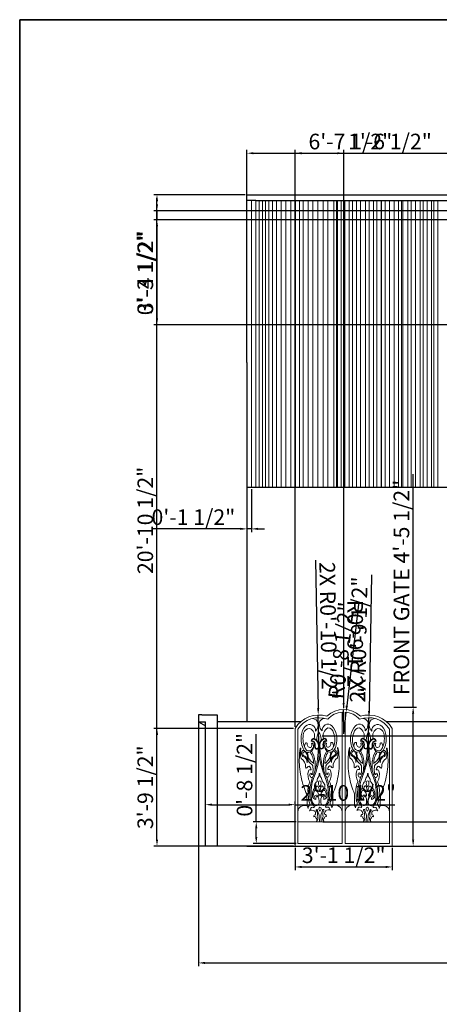
# Model space of a CAD drawing. Units: inches. Extents: x 2656 to 9931, y 1941 to 3068.
# Tile 28 of 46: x 2656 to 2817, y 2689 to 3068. Entities that reach past the tile are written whole.
import ezdxf

# ---------------------------------------------------------------- set-up
doc = ezdxf.new("R2010")
doc.units = ezdxf.units.IN
for name, color, linetype, lineweight in [('A-ANNO-DIMS', 2, 'Continuous', 18), ('A-ANNO-TTLB', 7, 'Continuous', 35), ('A-DOOR', 3, 'Continuous', 18), ('A-ELEV', 7, 'Continuous', 25), ('A-ELEV-FNSH', 8, 'Continuous', 13)]:
    doc.layers.add(name, color=color, linetype=linetype, lineweight=lineweight)
doc.styles.get("Standard").update_dxf_attribs({"font": 'arial.ttf'})
doc.dimstyles.new('ISO-25', dxfattribs={"dimtxt": 6, "dimasz": 2.5, "dimexe": 1.25, "dimexo": 0.625, "dimtad": 1, "dimdec": 0, "dimlunit": 3, "dimtxsty": 'Standard', "dimcen": 2.5, "dimadec": 0, "dimazin": 0, "dimtfac": 1, "dimtdec": 0, "dimtmove": 0, "dimatfit": 3, "dimfxl": 1, "dimarcsym": 0})

# ---------------------------------------------------------------- blocks, each defined once
blk = doc.blocks.new('A$C410F2A13')
for p, q in [((875, 2478), (875, 50)), ((925, 2478), (925, 50)), ((426, 2231), (424, 2281)), ((451, 2231), (449, 2281)), ((1349, 2231), (1351, 2281)), ((1374, 2231), (1376, 2281)), ((0, 2179), (0, 0)), ((50, 2165), (50, 50)), ((1750, 50), (1750, 2165)), ((1800, 0), (1800, 2179)), ((220, 960), (223, 746)), ((697, 967), (700, 754)), ((1103, 967), (1100, 754)), ((1580, 960), (1577, 746)), ((223, 746), (246, 699)), ((700, 754), (679, 706)), ((1100, 754), (1121, 706)), ((1577, 746), (1554, 699)), ((418, 661), (449, 574)), ((449, 574), (450, 450)), ((508, 662), (480, 574)), ((480, 574), (482, 450)), ((1292, 662), (1320, 574)), ((1320, 574), (1318, 450)), ((1351, 574), (1350, 450)), ((1382, 661), (1351, 574)), ((875, 450), (50, 450)), ((1750, 450), (925, 450)), ((1800, 0), (0, 0)), ((875, 50), (50, 50)), ((1750, 50), (925, 50))]:
    blk.add_line(p, q)
for centre, radius, start, end in [((440, 1914), 513, 72.8986, 148.9199), ((440, 1914), 463, 69.1804, 147.2414), ((900, 2081), 448, 46.332, 133.668), ((900, 2081), 398, 93.6017, 137.9637), ((900, 2081), 398, 42.0363, 86.3983), ((1360, 1914), 463, 32.7586, 110.8196), ((1360, 1914), 513, 31.0801, 107.1014), ((404, 2018), 289, 135.8089, 175.1456), ((271, 2143), 108, 353.1272, 134.3061), ((323, 2257), 103, 13.5799, 86.0018), ((283, 2236), 143, 311.7611, 357.9056), ((550, 2260), 103, 95.7845, 168.2064), ((594, 2241), 143, 183.8808, 230.0252), ((609, 2148), 108, 47.4802, 188.6591), ((683, 2044), 163, 118.0779, 198.0674), ((608, 2080), 107, 9.5072, 90.6984), ((433, 2000), 336, 8.9692, 42.4485), ((1367, 2000), 336, 137.5515, 171.0308), ((1192, 2080), 107, 89.3016, 170.4928), ((1191, 2148), 108, 351.3409, 132.5198), ((1117, 2044), 163, 341.9326, 61.9221), ((1250, 2260), 103, 11.7936, 84.2155), ((1206, 2241), 143, 309.9748, 356.1192), ((1517, 2236), 143, 182.0944, 228.2389), ((1477, 2257), 103, 93.9982, 166.4201), ((1529, 2143), 108, 45.6939, 186.8728), ((1396, 2018), 289, 4.8544, 44.1911), ((535, 1983), 424, 171.9264, 209.7222), ((548, 1989), 401, 165.5691, 203.7943), ((274, 2061), 118, 90.9442, 166.1424), ((206, 2037), 157, 343.347, 65.2388), ((652, 1980), 249, 148.1071, 184.9559), ((233, 1973), 249, 356.8304, 33.6792), ((397, 1973), 341, 336.2709, 21.5458), ((368, 1974), 405, 331.6018, 11.2466), ((1432, 1974), 405, 168.7534, 208.3982), ((1403, 1973), 341, 158.4542, 203.7291), ((1567, 1973), 249, 146.3208, 183.1696), ((1148, 1980), 249, 355.0441, 31.8929), ((1594, 2037), 157, 114.7612, 196.653), ((1526, 2061), 118, 13.8576, 89.0558), ((1252, 1989), 401, 336.2057, 14.4309), ((1265, 1983), 424, 330.2778, 8.0736), ((281, 1853), 103, 151.0965, 215.6191), ((208, 1894), 19.8, 343.1885, 153.073), ((277, 1877), 50.8, 167.4858, 297.2236), ((243, 1868), 67.5, 327.8515, 22.0134), ((345, 1949), 44.6, 75.3796, 190.4178), ((303, 1880), 60.3, 355.7551, 91.6639), ((320, 1892), 14.3, 341.4821, 176.919), ((215, 1844), 127, 316.4438, 20.3265), ((219, 1873), 125, 313.8899, 347.6181), ((345, 1949), 33.3, 46.9929, 175.401), ((303, 1880), 71.6, 354.0882, 82.8719), ((296, 1857), 147, 9.4138, 65.971), ((-859, 1778), 1310, 338.6825, 2.2697), ((540, 1859), 178, 174.573, 191.6445), ((405, 1834), 39.9, 195.7675, 306.6665), ((296, 1857), 136, 9.1053, 58.3227), ((540, 1859), 167, 175.2094, 191.4957), ((405, 1834), 28.6, 196.5254, 303.426), ((356, 1855), 78.9, 325.1027, 17.281), ((356, 1855), 90.2, 323.8055, 16.7629), ((1750, 1819), 1310, 179.8498, 203.1038), ((536, 1858), 90.2, 165.0234, 217.9808), ((595, 1862), 147, 115.8153, 172.3725), ((536, 1858), 78.9, 164.5053, 216.6837), ((595, 1862), 136, 123.4636, 172.681), ((488, 1835), 39.9, 235.1198, 346.0188), ((488, 1835), 28.6, 238.3603, 345.2609), ((351, 1856), 167, 350.2906, 6.5769), ((587, 1885), 71.6, 98.9144, 187.6981), ((543, 1952), 33.3, 6.3853, 134.7934), ((351, 1856), 178, 350.1418, 7.2133), ((587, 1885), 60.3, 90.1225, 186.0313), ((543, 1952), 44.6, 351.3685, 106.4067), ((675, 1851), 127, 161.4598, 225.3425), ((670, 1880), 125, 194.1682, 227.8964), ((568, 1896), 14.3, 4.8673, 200.3042), ((645, 1874), 67.5, 159.773, 213.9348), ((611, 1882), 50.8, 244.5627, 14.3005), ((679, 1901), 19.8, 28.7133, 198.5978), ((608, 1858), 103, 326.1672, 30.6898), ((790, 1818), 4.67, 13.9519, 189.3402), ((1010, 1818), 4.67, 350.6598, 166.0481), ((1192, 1858), 103, 149.3102, 213.8328), ((1121, 1901), 19.8, 341.4022, 151.2867), ((1189, 1882), 50.8, 165.6995, 295.4373), ((1155, 1874), 67.5, 326.0652, 20.227), ((1257, 1952), 44.6, 73.5933, 188.6315), ((1213, 1885), 60.3, 353.9687, 89.8775), ((1125, 1851), 127, 314.6575, 18.5402), ((1130, 1880), 125, 312.1036, 345.8318), ((1232, 1896), 14.3, 339.6958, 175.1327), ((1257, 1952), 33.3, 45.2066, 173.6147), ((1213, 1885), 71.6, 352.3019, 81.0856), ((50, 1819), 1310, 336.8962, 0.1502), ((1205, 1862), 147, 7.6275, 64.1847), ((1449, 1856), 178, 172.7867, 189.8582), ((1312, 1835), 39.9, 193.9812, 304.8802), ((1205, 1862), 136, 7.319, 56.5364), ((1449, 1856), 167, 173.4231, 189.7094), ((1312, 1835), 28.6, 194.7391, 301.6397), ((1264, 1858), 78.9, 323.3163, 15.4947), ((1264, 1858), 90.2, 322.0192, 14.9766), ((2659, 1778), 1310, 177.7303, 201.3175), ((1444, 1855), 90.2, 163.2371, 216.1945), ((1504, 1857), 147, 114.029, 170.5862), ((1444, 1855), 78.9, 162.719, 214.8973), ((1504, 1857), 136, 121.6773, 170.8947), ((1395, 1834), 39.9, 233.3335, 344.2325), ((1395, 1834), 28.6, 236.574, 343.4746), ((1260, 1859), 167, 348.5043, 4.7906), ((1497, 1880), 71.6, 97.1281, 185.9118), ((1455, 1949), 33.3, 4.599, 133.0071), ((1260, 1859), 178, 348.3555, 5.427), ((1497, 1880), 60.3, 88.3361, 184.2449), ((1455, 1949), 44.6, 349.5822, 104.6204), ((1585, 1844), 127, 159.6735, 223.5562), ((1581, 1873), 125, 192.3819, 226.1101), ((1480, 1892), 14.3, 3.081, 198.5179), ((1557, 1868), 67.5, 157.9866, 212.1485), ((1523, 1877), 50.8, 242.7764, 12.5142), ((1592, 1894), 19.8, 26.927, 196.8115), ((1519, 1853), 103, 324.3809, 28.9035), ((1612, 1585), 1533, 171.6093, 184.3031), ((100, 1808), 4.67, 352.4461, 167.8344), ((541, 1734), 442, 170.4372, 194.6126), ((203, 1716), 81.7, 156.3863, 223.0742), ((160, 1741), 32.3, 77.4748, 166.6263), ((182, 1708), 40.1, 125.8941, 234.0122), ((120, 1560), 103, 350.7161, 76.6459), ((177, 1718), 29.4, 30.9708, 129.0147), ((137, 1589), 89.3, 5.6042, 76.0929), ((251, 1839), 107, 218.4659, 256.4745), ((256, 1836), 73, 216.1033, 312.5948), ((86, 1643), 147, 341.991, 37.7938), ((242, 1834), 101, 260.608, 309.4662), ((-8, 1638), 253, 349.0382, 22.4521), ((537, 1793), 328, 207.3657, 234.2277), ((6, 1539), 339, 357.9888, 36.5364), ((-43, 1535), 413, 5.2421, 32.4725), ((-859, 1778), 1288, 338.6825, 1.0491), ((1750, 1819), 1288, 180.5839, 203.1038), ((941, 1550), 413, 149.3138, 176.5442), ((892, 1552), 339, 145.2499, 183.7975), ((354, 1790), 328, 307.5586, 334.4207), ((633, 1842), 73, 229.1915, 325.6831), ((647, 1841), 101, 232.3202, 281.1783), ((904, 1653), 253, 159.3342, 192.7481), ((809, 1654), 147, 143.9925, 199.7953), ((638, 1845), 107, 285.3118, 323.3204), ((760, 1599), 89.3, 105.6934, 176.1821), ((778, 1570), 103, 105.1404, 191.0702), ((716, 1726), 29.4, 52.7716, 150.8155), ((732, 1750), 32.3, 15.16, 104.3116), ((712, 1716), 40.1, 307.7741, 55.8923), ((690, 1723), 81.7, 318.7122, 25.4), ((352, 1731), 442, 347.1737, 11.3491), ((-714, 1549), 1533, 357.4832, 10.177), ((2514, 1549), 1533, 169.823, 182.5168), ((1448, 1731), 442, 168.6509, 192.8263), ((1110, 1723), 81.7, 154.6, 221.2878), ((1068, 1750), 32.3, 75.6884, 164.84), ((1088, 1716), 40.1, 124.1077, 232.2259), ((1022, 1570), 103, 348.9298, 74.8596), ((1040, 1599), 89.3, 3.8179, 74.3066), ((1084, 1726), 29.4, 29.1845, 127.2284), ((1162, 1845), 107, 216.6796, 254.6882), ((1167, 1842), 73, 214.3169, 310.8085), ((991, 1654), 147, 340.2047, 36.0075), ((1153, 1841), 101, 258.8217, 307.6798), ((896, 1653), 253, 347.2519, 20.6658), ((1446, 1790), 328, 205.5793, 232.4414), ((908, 1552), 339, 356.2025, 34.7501), ((859, 1550), 413, 3.4558, 30.6862), ((50, 1819), 1288, 336.8962, 359.4161), ((2659, 1778), 1288, 178.9509, 201.3175), ((1843, 1535), 413, 147.5275, 174.7579), ((1794, 1539), 339, 143.4636, 182.0112), ((1263, 1793), 328, 305.7723, 332.6343), ((1544, 1836), 73, 227.4052, 323.8967), ((1558, 1834), 101, 230.5338, 279.392), ((1808, 1638), 253, 157.5479, 190.9618), ((1714, 1643), 147, 142.2062, 198.009), ((1549, 1839), 107, 283.5255, 321.5341), ((1663, 1589), 89.3, 103.9071, 174.3958), ((1680, 1560), 103, 103.3541, 189.2839), ((1623, 1718), 29.4, 50.9853, 149.0292), ((1640, 1741), 32.3, 13.3737, 102.5252), ((1618, 1708), 40.1, 305.9878, 54.1059), ((1597, 1716), 81.7, 316.9258, 23.6137), ((1259, 1734), 442, 345.3874, 9.5628), ((1700, 1808), 4.67, 12.1656, 187.5539), ((188, 1585), 1533, 355.6969, 8.3907), ((1515, 1588), 1436, 184.7143, 199.6369), ((20, 1472), 176, 356.4272, 58.168), ((211, 1459), 15, 168.6782, 347.0514), ((289, 1544), 66.9, 136.2114, 182.0632), ((276, 1426), 58.2, 104.7242, 150.243), ((355, 1631), 122, 199.5388, 236.1164), ((215, 1415), 81.6, 357.4438, 55.6636), ((252, 1458), 79.7, 3.4811, 64.0466), ((-203, 1415), 537, 351.9282, 5.1024), ((-1131, 1472), 1504, 357.1404, 3.8345), ((2032, 1521), 1504, 177.9518, 184.6459), ((1105, 1436), 537, 176.6839, 189.8581), ((649, 1464), 79.7, 117.7397, 178.3052), ((688, 1423), 81.6, 126.1227, 184.3425), ((541, 1634), 122, 305.6699, 342.2475), ((626, 1432), 58.2, 31.5433, 77.0621), ((610, 1549), 66.9, 359.7232, 45.5749), ((691, 1466), 15, 194.7349, 13.1081), ((881, 1486), 176, 123.6183, 185.3591), ((-788, 1575), 1608, 343.3715, 356.674), ((2588, 1575), 1608, 183.326, 196.6285), ((919, 1486), 176, 354.6409, 56.3817), ((1109, 1466), 15, 166.8919, 345.2651), ((1190, 1549), 66.9, 134.4251, 180.2768), ((1174, 1432), 58.2, 102.9379, 148.4567), ((1259, 1634), 122, 197.7525, 234.3301), ((1112, 1423), 81.6, 355.6575, 53.8773), ((1151, 1464), 79.7, 1.6948, 62.2603), ((695, 1436), 537, 350.1419, 3.3161), ((-232, 1521), 1504, 355.3541, 2.0482), ((2931, 1472), 1504, 176.1655, 182.8596), ((2003, 1415), 537, 174.8976, 188.0718), ((1548, 1458), 79.7, 115.9534, 176.5189), ((1585, 1415), 81.6, 124.3364, 182.5562), ((1445, 1631), 122, 303.8836, 340.4612), ((1524, 1426), 58.2, 29.757, 75.2758), ((1511, 1544), 66.9, 357.9368, 43.7886), ((1589, 1459), 15, 192.9486, 11.3218), ((1780, 1472), 176, 121.832, 183.5728), ((285, 1588), 1436, 340.3631, 355.2857), ((510, 1325), 272, 165.7404, 209.4263), ((282, 1375), 39.5, 68.6283, 153.8782), ((335, 1320), 60.6, 168.2152, 221.9825), ((1112, 984), 838, 157.0956, 187.6467), ((294, 1332), 18.8, 3.4092, 180.1447), ((308, 1293), 23.3, 216.4325, 342.6737), ((1112, 984), 815, 157.0956, 187.6467), ((308, 1329), 6.31, 42.5614, 221.6206), ((311, 1341), 17.8, 245.7105, 355.9064), ((375, 1323), 72.5, 313.9549, 9.9508), ((453, 1336), 6.37, 351.4407, 190.3456), ((531, 1325), 72.5, 171.8355, 227.8314), ((-196, 964), 815, 354.1396, 24.6908), ((-196, 964), 838, 354.1396, 24.6908), ((594, 1346), 17.8, 185.8799, 296.0758), ((598, 1298), 23.3, 199.1126, 325.3538), ((611, 1337), 18.8, 1.6416, 178.3771), ((597, 1334), 6.31, 320.1657, 139.2249), ((622, 1380), 39.5, 27.9081, 113.158), ((571, 1324), 60.6, 319.8038, 13.5711), ((396, 1323), 272, 332.36, 16.0459), ((1404, 1323), 272, 163.9541, 207.64), ((1178, 1380), 39.5, 66.842, 152.0919), ((1996, 964), 838, 155.3092, 185.8604), ((1229, 1324), 60.6, 166.4289, 220.1962), ((1189, 1337), 18.8, 1.6229, 178.3584), ((1996, 964), 815, 155.3092, 185.8604), ((1202, 1298), 23.3, 214.6462, 340.8874), ((1203, 1334), 6.31, 40.7751, 219.8343), ((1206, 1346), 17.8, 243.9242, 354.1201), ((1269, 1325), 72.5, 312.1686, 8.1645), ((1347, 1336), 6.37, 349.6544, 188.5593), ((1425, 1323), 72.5, 170.0492, 226.0451), ((688, 984), 815, 352.3533, 22.9044), ((688, 984), 838, 352.3533, 22.9044), ((1492, 1293), 23.3, 197.3263, 323.5675), ((1489, 1341), 17.8, 184.0936, 294.2895), ((1506, 1332), 18.8, 359.8553, 176.5908), ((1492, 1329), 6.31, 318.3794, 137.4386), ((1518, 1375), 39.5, 26.1218, 111.3717), ((1465, 1320), 60.6, 318.0175, 11.7848), ((1290, 1325), 272, 330.5737, 14.2596), ((1034, 1366), 910, 196.6416, 206.516), ((651, 1026), 412, 156.3521, 186.153), ((460, 1109), 99.3, 121.7041, 214.2648), ((432, 1077), 42.5, 130.9198, 211.0137), ((413, 1099), 13.8, 29.7957, 133.7989), ((543, 1204), 135, 150.4288, 184.5495), ((296, 1026), 152, 352.3578, 31.816), ((548, 1163), 114, 168.6269, 216.6185), ((458, 1185), 22, 10.8248, 177.088), ((359, 1169), 122, 322.7993, 9.2913), ((618, 1031), 152, 149.9703, 189.4285), ((366, 1201), 135, 357.2368, 31.3575), ((499, 1100), 13.8, 47.9874, 151.9906), ((452, 1108), 99.3, 327.5215, 60.0822), ((482, 1078), 42.5, 330.7726, 50.8665), ((264, 1020), 412, 355.6333, 25.4342), ((-228, 1401), 1022, 334.8573, 343.6994), ((2028, 1401), 1022, 196.3006, 205.1427), ((1536, 1020), 412, 154.5658, 184.3667), ((1348, 1108), 99.3, 119.9178, 212.4785), ((1318, 1078), 42.5, 129.1335, 209.2274), ((1301, 1100), 13.8, 28.0094, 132.0126), ((1434, 1201), 135, 148.6425, 182.7632), ((1182, 1031), 152, 350.5715, 30.0297), ((1441, 1169), 122, 170.7087, 217.2007), ((1342, 1185), 22, 2.912, 169.1752), ((1252, 1163), 114, 323.3815, 11.3731), ((1504, 1026), 152, 148.184, 187.6422), ((1257, 1204), 135, 355.4505, 29.5712), ((1387, 1099), 13.8, 46.2011, 150.2043), ((1340, 1109), 99.3, 325.7352, 58.2959), ((1368, 1077), 42.5, 328.9863, 49.0802), ((1149, 1026), 412, 353.847, 23.6479), ((766, 1366), 910, 333.484, 343.3584), ((-1225, 770), 1481, 2.6409, 8.2601), ((514, 961), 194, 154.3669, 193.8901), ((392, 933), 69.6, 195.2601, 265.1721), ((361, 1035), 24.7, 46.0398, 154.5946), ((446, 964), 104, 145.8083, 215.978), ((378, 1011), 22, 40.8296, 145.9256), ((407, 900), 45.3, 101.6882, 175.5), ((451, 879), 66.5, 145.8201, 193.29), ((321, 927), 122, 357.8138, 53.2441), ((510, 1123), 133, 210.7996, 241.8374), ((409, 896), 23.8, 28.136, 121.6978), ((401, 892), 51.9, 35.6248, 94.1694), ((402, 1121), 133, 299.949, 330.9867), ((597, 931), 122, 128.5422, 183.9725), ((518, 894), 51.9, 87.6169, 146.1615), ((510, 898), 23.8, 60.0886, 153.6503), ((538, 1013), 22, 35.8607, 140.9567), ((512, 901), 45.3, 6.2863, 80.0981), ((468, 879), 66.5, 348.4963, 35.9662), ((525, 935), 69.6, 276.6142, 346.5263), ((553, 1038), 24.7, 27.1917, 135.7465), ((471, 965), 104, 325.8083, 35.978), ((403, 960), 194, 347.8962, 27.4194), ((2146, 822), 1481, 173.5262, 179.1454), ((-346, 822), 1481, 0.8546, 6.4738), ((1397, 960), 194, 152.5806, 192.1038), ((1275, 935), 69.6, 193.4737, 263.3858), ((1247, 1038), 24.7, 44.2535, 152.8083), ((1329, 965), 104, 144.022, 214.1917), ((1288, 901), 45.3, 99.9019, 173.7137), ((1262, 1013), 22, 39.0433, 144.1393), ((1332, 879), 66.5, 144.0338, 191.5037), ((1290, 898), 23.8, 26.3497, 119.9114), ((1203, 931), 122, 356.0275, 51.4578), ((1282, 894), 51.9, 33.8385, 92.3831), ((1398, 1121), 133, 209.0133, 240.051), ((1290, 1123), 133, 298.1626, 329.2004), ((1479, 927), 122, 126.7559, 182.1862), ((1399, 892), 51.9, 85.8306, 144.3752), ((1391, 896), 23.8, 58.3022, 151.864), ((1393, 900), 45.3, 4.5, 78.3118), ((1349, 879), 66.5, 346.71, 34.1799), ((1422, 1011), 22, 34.0744, 139.1704), ((1408, 933), 69.6, 274.8279, 344.7399), ((1439, 1035), 24.7, 25.4054, 133.9602), ((1354, 964), 104, 324.022, 34.1917), ((1286, 961), 194, 346.1099, 25.6331), ((3025, 770), 1481, 171.7399, 177.3591), ((178, 627), 128, 69.0706, 176.8846), ((308, 708), 62.6, 122.2779, 188.4961), ((126, 764), 148, 358.7797, 29.7342), ((489, 897), 208, 186.6395, 229.065), ((489, 897), 186, 186.6395, 229.065), ((344, 728), 14.3, 246.7853, 56.0942), ((395, 798), 50.3, 236.3592, 331.1413), ((211, 825), 234, 347.3605, 20.5181), ((710, 833), 234, 161.2682, 194.4258), ((527, 801), 50.3, 210.645, 305.4271), ((430, 896), 186, 312.7213, 355.1469), ((580, 731), 14.3, 125.6921, 295.001), ((430, 896), 208, 312.7213, 355.1469), ((797, 775), 148, 152.0521, 183.0067), ((617, 713), 62.6, 353.2902, 59.5084), ((738, 622), 137, 5.1669, 105.9832), ((1062, 622), 137, 74.0168, 174.8331), ((1183, 713), 62.6, 120.4916, 186.7098), ((1003, 775), 148, 356.9933, 27.9479), ((1370, 896), 208, 184.8531, 227.2787), ((1370, 896), 186, 184.8531, 227.2787), ((1220, 731), 14.3, 244.999, 54.3079), ((1273, 801), 50.3, 234.5729, 329.355), ((1090, 833), 234, 345.5742, 18.7318), ((1589, 825), 234, 159.4819, 192.6395), ((1405, 798), 50.3, 208.8587, 303.6408), ((1311, 897), 186, 310.935, 353.3605), ((1456, 728), 14.3, 123.9058, 293.2147), ((1311, 897), 208, 310.935, 353.3605), ((1674, 764), 148, 150.2658, 181.2203), ((1492, 708), 62.6, 351.5039, 57.7221), ((1622, 627), 128, 3.1154, 110.9294), ((240, 690), 44.7, 310.1016, 354.7847), ((309, 568), 96.9, 61.1389, 114.4638), ((322, 681), 37.3, 63.2668, 172.2295), ((377, 551), 31.2, 88.6919, 191.8345), ((360, 526), 23.2, 351.6032, 126.2426), ((319, 603), 62.5, 340.859, 53.3331), ((406, 663), 12.7, 349.8969, 198.3449), ((302, 590), 115, 338.9282, 37.0597), ((354, 505), 70.4, 316.5398, 37.6736), ((462, 695), 23.7, 13.2533, 176.8954), ((503, 699), 64.1, 181.769, 232.1167), ((411, 701), 74.6, 314.8438, 359.9081), ((577, 508), 70.4, 144.1128, 225.2465), ((520, 665), 12.7, 343.4414, 191.8894), ((627, 595), 115, 144.7267, 202.8581), ((609, 607), 62.5, 128.4533, 200.9273), ((570, 529), 23.2, 55.5438, 190.1831), ((553, 554), 31.2, 349.9518, 93.0944), ((620, 573), 96.9, 67.3225, 120.6474), ((604, 686), 37.3, 9.5569, 118.5195), ((685, 697), 44.7, 187.0016, 231.6847), ((1115, 697), 44.7, 308.3153, 352.9984), ((1180, 573), 96.9, 59.3526, 112.6775), ((1196, 686), 37.3, 61.4805, 170.4431), ((1247, 554), 31.2, 86.9056, 190.0482), ((1230, 529), 23.2, 349.8169, 124.4562), ((1191, 607), 62.5, 339.0727, 51.5467), ((1280, 665), 12.7, 348.1106, 196.5586), ((1173, 595), 115, 337.1419, 35.2733), ((1223, 508), 70.4, 314.7535, 35.8872), ((1338, 695), 23.7, 3.1046, 166.7467), ((1389, 701), 74.6, 180.0919, 225.1562), ((1297, 699), 64.1, 307.8833, 358.231), ((1446, 505), 70.4, 142.3264, 223.4602), ((1394, 663), 12.7, 341.6551, 190.1031), ((1498, 590), 115, 142.9403, 201.0718), ((1440, 526), 23.2, 53.7574, 188.3968), ((1481, 603), 62.5, 126.6669, 199.141), ((1423, 551), 31.2, 348.1655, 91.3081), ((1491, 568), 96.9, 65.5362, 118.8611), ((1478, 681), 37.3, 7.7705, 116.7332), ((1560, 690), 44.7, 185.2153, 229.8984), ((356, 484), 47.1, 328.1103, 55.2335), ((401, 458), 4.38, 168.7041, 339.394), ((575, 487), 47.1, 126.5529, 213.676), ((532, 460), 4.38, 202.3923, 13.0822), ((1225, 487), 47.1, 326.324, 53.4471), ((1268, 460), 4.38, 166.9178, 337.6077), ((1399, 458), 4.38, 200.606, 11.2959), ((1444, 484), 47.1, 124.7665, 211.8897)]:
    blk.add_arc(centre, radius, start, end)
blk = doc.blocks.new('*D63')
at = {"layer": 'A-ANNO-DIMS', "color": 0, "lineweight": -2, "transparency": 16777216}
for p, q in [((2807.09, 2803.32), (2807.09, 2893)), ((2799.7, 2803.32), (2808.34, 2803.32)), ((2807.09, 2752.39), (2807.09, 2800.82)), ((2799.7, 2749.89), (2808.34, 2749.89))]:
    blk.add_line(p, q, dxfattribs=at)
at = {"layer": 'A-ANNO-DIMS', "color": 0, "transparency": 16777216}
for points in [[(2806.67, 2800.82), (2807.5, 2800.82), (2807.09, 2803.32)], [(2806.67, 2752.39), (2807.5, 2752.39), (2807.09, 2749.89)]]:
    blk.add_solid(points, dxfattribs=at)
at = {"layer": 'Defpoints', "color": 0, "transparency": 16777216}
for p in [(2799.07, 2803.32), (2807.09, 2803.32), (2799.07, 2749.89)]:
    blk.add_point(p, dxfattribs=at)
at = {"layer": 'A-ANNO-DIMS', "color": 0, "transparency": 16777216, "insert": (2803.36, 2849.41), "char_height": 6, "attachment_point": 5, "rotation": 90}
blk.add_mtext('FRONT GATE 4\'-5 1/2"', dxfattribs=at)
blk = doc.blocks.new('*D64')
at = {"layer": 'A-ANNO-DIMS', "color": 0, "lineweight": -2, "transparency": 16777216}
for p, q in [((2761.66, 2749.27), (2761.66, 2740.63)), ((2799.07, 2749.27), (2799.07, 2740.63)), ((2764.16, 2741.88), (2796.57, 2741.88))]:
    blk.add_line(p, q, dxfattribs=at)
at = {"layer": 'A-ANNO-DIMS', "color": 0, "transparency": 16777216}
for points in [[(2764.16, 2742.3), (2764.16, 2741.46), (2761.66, 2741.88)], [(2796.57, 2742.3), (2796.57, 2741.46), (2799.07, 2741.88)]]:
    blk.add_solid(points, dxfattribs=at)
at = {"layer": 'Defpoints', "color": 0, "transparency": 16777216}
for p in [(2761.66, 2749.89), (2799.07, 2749.89), (2799.07, 2741.88)]:
    blk.add_point(p, dxfattribs=at)
at = {"layer": 'A-ANNO-DIMS', "color": 0, "transparency": 16777216, "insert": (2780.37, 2745.61), "char_height": 6, "attachment_point": 5}
blk.add_mtext('3\'-1 1/2"', dxfattribs=at)
blk = doc.blocks.new('*D77')
at = {"layer": 'A-ANNO-DIMS', "color": 0, "lineweight": -2, "transparency": 16777216}
for p, q in [((2724.52, 2799.77), (2724.52, 2703.71)), ((3030.16, 2801), (3030.16, 2703.71)), ((2727.02, 2704.96), (3027.66, 2704.96))]:
    blk.add_line(p, q, dxfattribs=at)
at = {"layer": 'A-ANNO-DIMS', "color": 0, "transparency": 16777216}
for points in [[(2727.02, 2705.38), (2727.02, 2704.54), (2724.52, 2704.96)], [(3027.66, 2705.38), (3027.66, 2704.54), (3030.16, 2704.96)]]:
    blk.add_solid(points, dxfattribs=at)
at = {"layer": 'Defpoints', "color": 0, "transparency": 16777216}
for p in [(2724.52, 2800.4), (3030.16, 2801.62), (3030.16, 2704.96)]:
    blk.add_point(p, dxfattribs=at)
at = {"layer": 'A-ANNO-DIMS', "color": 0, "transparency": 16777216, "insert": (2877.34, 2708.69), "char_height": 6, "attachment_point": 5}
blk.add_mtext('25\'-5 1/2"', dxfattribs=at)
blk = doc.blocks.new('*D78')
at = {"layer": 'A-ANNO-DIMS', "color": 0, "lineweight": -2, "transparency": 16777216}
for p, q in [((2742.53, 3000.52), (2707.32, 3000.52)), ((2708.57, 2752.39), (2708.57, 2998.02)), ((2726.57, 2749.89), (2707.32, 2749.89))]:
    blk.add_line(p, q, dxfattribs=at)
at = {"layer": 'A-ANNO-DIMS', "color": 0, "transparency": 16777216}
for points in [[(2708.16, 2998.02), (2708.99, 2998.02), (2708.57, 3000.52)], [(2708.16, 2752.39), (2708.99, 2752.39), (2708.57, 2749.89)]]:
    blk.add_solid(points, dxfattribs=at)
at = {"layer": 'Defpoints', "color": 0, "transparency": 16777216}
for p in [(2708.57, 3000.52), (2743.16, 3000.52), (2727.19, 2749.89)]:
    blk.add_point(p, dxfattribs=at)
at = {"layer": 'A-ANNO-DIMS', "color": 0, "transparency": 16777216, "insert": (2704.85, 2875.21), "char_height": 6, "attachment_point": 5, "rotation": 90}
blk.add_mtext('20\'-10 1/2"', dxfattribs=at)
blk = doc.blocks.new('*D83')
at = {"layer": 'A-ANNO-DIMS', "color": 0, "lineweight": -2, "transparency": 16777216}
for p, q in [((2743.16, 2998.91), (2743.16, 3017.72)), ((2745.66, 3016.47), (2820.21, 3016.47)), ((2822.71, 2998.91), (2822.71, 3017.72))]:
    blk.add_line(p, q, dxfattribs=at)
at = {"layer": 'A-ANNO-DIMS', "color": 0, "transparency": 16777216}
for points in [[(2745.66, 3016.88), (2745.66, 3016.05), (2743.16, 3016.47)], [(2820.21, 3016.88), (2820.21, 3016.05), (2822.71, 3016.47)]]:
    blk.add_solid(points, dxfattribs=at)
at = {"layer": 'Defpoints', "color": 0, "transparency": 16777216}
for p in [(2822.71, 3016.47), (2743.16, 2998.29), (2822.71, 2998.29)]:
    blk.add_point(p, dxfattribs=at)
at = {"layer": 'A-ANNO-DIMS', "color": 0, "transparency": 16777216, "insert": (2782.93, 3020.19), "char_height": 6, "attachment_point": 5}
blk.add_mtext('6\'-7 1/2"', dxfattribs=at)
blk = doc.blocks.new('*D88')
at = {"layer": 'A-ANNO-DIMS', "color": 0, "lineweight": -2, "transparency": 16777216}
for p, q in [((2727.19, 2750.52), (2727.19, 2767.09)), ((2729.69, 2765.84), (2759.16, 2765.84)), ((2761.66, 2750.52), (2761.66, 2767.09)), ((2761.66, 2765.84), (2800.1, 2765.84))]:
    blk.add_line(p, q, dxfattribs=at)
at = {"layer": 'A-ANNO-DIMS', "color": 0, "transparency": 16777216}
for points in [[(2729.69, 2766.26), (2729.69, 2765.43), (2727.19, 2765.84)], [(2759.16, 2766.26), (2759.16, 2765.43), (2761.66, 2765.84)]]:
    blk.add_solid(points, dxfattribs=at)
at = {"layer": 'Defpoints', "color": 0, "transparency": 16777216}
for p in [(2761.66, 2765.84), (2727.19, 2749.89), (2761.66, 2749.89)]:
    blk.add_point(p, dxfattribs=at)
at = {"layer": 'A-ANNO-DIMS', "color": 0, "transparency": 16777216, "insert": (2782.13, 2769.57), "char_height": 6, "attachment_point": 5}
blk.add_mtext('2\'-10 1/2"', dxfattribs=at)
blk = doc.blocks.new('*D152')
at = {"layer": 'A-ANNO-DIMS', "color": 0, "lineweight": -2, "transparency": 16777216}
for p, q in [((2847.28, 2990.83), (2707.32, 2990.83)), ((2708.57, 2988.33), (2708.57, 2952.97)), ((2847.25, 2950.47), (2707.32, 2950.47))]:
    blk.add_line(p, q, dxfattribs=at)
at = {"layer": 'A-ANNO-DIMS', "color": 0, "transparency": 16777216}
for points in [[(2708.16, 2988.33), (2708.99, 2988.33), (2708.57, 2990.83)], [(2708.16, 2952.97), (2708.99, 2952.97), (2708.57, 2950.47)]]:
    blk.add_solid(points, dxfattribs=at)
at = {"layer": 'Defpoints', "color": 0, "transparency": 16777216}
for p in [(2847.9, 2990.83), (2708.57, 2950.47), (2847.87, 2950.47)]:
    blk.add_point(p, dxfattribs=at)
at = {"layer": 'A-ANNO-DIMS', "color": 0, "transparency": 16777216, "insert": (2704.84, 2970.65), "char_height": 6, "attachment_point": 5, "rotation": 90}
blk.add_mtext('3\'-4 1/2"', dxfattribs=at)
blk = doc.blocks.new('*D154')
at = {"layer": 'A-ANNO-DIMS', "color": 0, "lineweight": -2, "transparency": 16777216}
for p, q in [((2708.57, 2996.85), (2708.57, 2999.35)), ((2826.02, 2994.35), (2707.32, 2994.35)), ((2708.57, 2994.35), (2708.57, 2990.83)), ((2847.28, 2990.83), (2707.32, 2990.83)), ((2708.57, 2988.33), (2708.57, 2954.65))]:
    blk.add_line(p, q, dxfattribs=at)
at = {"layer": 'A-ANNO-DIMS', "color": 0, "transparency": 16777216}
for points in [[(2708.16, 2996.85), (2708.99, 2996.85), (2708.57, 2994.35)], [(2708.16, 2988.33), (2708.99, 2988.33), (2708.57, 2990.83)]]:
    blk.add_solid(points, dxfattribs=at)
at = {"layer": 'Defpoints', "color": 0, "transparency": 16777216}
for p in [(2826.64, 2994.35), (2708.57, 2990.83), (2847.9, 2990.83)]:
    blk.add_point(p, dxfattribs=at)
at = {"layer": 'A-ANNO-DIMS', "color": 0, "transparency": 16777216, "insert": (2704.84, 2970.24), "char_height": 6, "attachment_point": 5, "rotation": 90}
blk.add_mtext('0\'-3 1/2"', dxfattribs=at)
blk = doc.blocks.new('*D155')
at = {"layer": 'A-ANNO-DIMS', "color": 0, "lineweight": -2, "transparency": 16777216}
for p, q in [((2743.16, 2887.27), (2743.16, 2870.69)), ((2744.89, 2887.27), (2744.89, 2870.69)), ((2740.66, 2871.94), (2706.98, 2871.94)), ((2744.89, 2871.94), (2743.16, 2871.94)), ((2747.39, 2871.94), (2749.89, 2871.94))]:
    blk.add_line(p, q, dxfattribs=at)
at = {"layer": 'A-ANNO-DIMS', "color": 0, "transparency": 16777216}
for points in [[(2740.66, 2872.36), (2740.66, 2871.53), (2743.16, 2871.94)], [(2747.39, 2872.36), (2747.39, 2871.53), (2744.89, 2871.94)]]:
    blk.add_solid(points, dxfattribs=at)
at = {"layer": 'Defpoints', "color": 0, "transparency": 16777216}
for p in [(2743.16, 2887.89), (2744.89, 2887.89), (2743.16, 2871.94)]:
    blk.add_point(p, dxfattribs=at)
at = {"layer": 'A-ANNO-DIMS', "color": 0, "transparency": 16777216, "insert": (2722.57, 2875.67), "char_height": 6, "attachment_point": 5}
blk.add_mtext('0\'-1 1/2"', dxfattribs=at)
blk = doc.blocks.new('*D169')
at = {"layer": 'A-ANNO-DIMS', "color": 0, "lineweight": -2, "transparency": 16777216}
for p, q in [((2761.03, 2795.19), (2707.32, 2795.19)), ((2708.57, 2752.39), (2708.57, 2792.69)), ((2761.03, 2749.89), (2707.32, 2749.89))]:
    blk.add_line(p, q, dxfattribs=at)
at = {"layer": 'A-ANNO-DIMS', "color": 0, "transparency": 16777216}
for points in [[(2708.16, 2792.69), (2708.99, 2792.69), (2708.57, 2795.19)], [(2708.16, 2752.39), (2708.99, 2752.39), (2708.57, 2749.89)]]:
    blk.add_solid(points, dxfattribs=at)
at = {"layer": 'Defpoints', "color": 0, "transparency": 16777216}
for p in [(2708.57, 2795.19), (2761.66, 2795.19), (2761.66, 2749.89)]:
    blk.add_point(p, dxfattribs=at)
at = {"layer": 'A-ANNO-DIMS', "color": 0, "transparency": 16777216, "insert": (2704.84, 2772.54), "char_height": 6, "attachment_point": 5, "rotation": 90}
blk.add_mtext('3\'-9 1/2"', dxfattribs=at)
blk = doc.blocks.new('*D170')
at = {"layer": 'A-ANNO-DIMS', "color": 0, "lineweight": -2, "transparency": 16777216}
for p, q in [((2761.66, 2795.82), (2761.66, 3017.72)), ((2764.16, 3016.47), (2777.87, 3016.47)), ((2780.37, 2803.08), (2780.37, 3017.72)), ((2780.37, 3016.47), (2813.48, 3016.47))]:
    blk.add_line(p, q, dxfattribs=at)
at = {"layer": 'A-ANNO-DIMS', "color": 0, "transparency": 16777216}
for points in [[(2764.16, 3016.88), (2764.16, 3016.05), (2761.66, 3016.47)], [(2777.87, 3016.88), (2777.87, 3016.05), (2780.37, 3016.47)]]:
    blk.add_solid(points, dxfattribs=at)
at = {"layer": 'Defpoints', "color": 0, "transparency": 16777216}
for p in [(2780.37, 3016.47), (2780.37, 2802.46), (2761.66, 2795.19)]:
    blk.add_point(p, dxfattribs=at)
at = {"layer": 'A-ANNO-DIMS', "color": 0, "transparency": 16777216, "insert": (2798.17, 3020.19), "char_height": 6, "attachment_point": 5}
blk.add_mtext('1\'-6 1/2"', dxfattribs=at)
blk = doc.blocks.new('*D171')
at = {"layer": 'A-ANNO-DIMS', "color": 0, "lineweight": -2, "transparency": 16777216}
for p, q in [((2746.75, 2759.25), (2746.75, 2792.93)), ((2762.07, 2759.25), (2745.5, 2759.25)), ((2746.75, 2753.43), (2746.75, 2756.75)), ((2762.07, 2750.93), (2745.5, 2750.93))]:
    blk.add_line(p, q, dxfattribs=at)
at = {"layer": 'A-ANNO-DIMS', "color": 0, "transparency": 16777216}
for points in [[(2746.33, 2756.75), (2747.16, 2756.75), (2746.75, 2759.25)], [(2746.33, 2753.43), (2747.16, 2753.43), (2746.75, 2750.93)]]:
    blk.add_solid(points, dxfattribs=at)
at = {"layer": 'Defpoints', "color": 0, "transparency": 16777216}
for p in [(2746.75, 2759.25), (2762.7, 2759.25), (2762.7, 2750.93)]:
    blk.add_point(p, dxfattribs=at)
at = {"layer": 'A-ANNO-DIMS', "color": 0, "transparency": 16777216, "insert": (2743.02, 2777.34), "char_height": 6, "attachment_point": 5, "rotation": 90}
blk.add_mtext('0\'-8 1/2"', dxfattribs=at)
blk = doc.blocks.new('*D179')
at = {"layer": 'A-ANNO-DIMS', "color": 0, "lineweight": -2, "transparency": 16777216}
for p, q in [((2772.12, 2792.27), (3047.36, 2792.27)), ((3046.11, 2761.76), (3046.11, 2789.77)), ((2772.31, 2759.26), (3047.36, 2759.26))]:
    blk.add_line(p, q, dxfattribs=at)
at = {"layer": 'A-ANNO-DIMS', "color": 0, "transparency": 16777216}
for points in [[(3045.69, 2789.77), (3046.53, 2789.77), (3046.11, 2792.27)], [(3045.69, 2761.76), (3046.53, 2761.76), (3046.11, 2759.26)]]:
    blk.add_solid(points, dxfattribs=at)
at = {"layer": 'Defpoints', "color": 0, "transparency": 16777216}
for p in [(2771.5, 2792.27), (3046.11, 2792.27), (2771.68, 2759.26)]:
    blk.add_point(p, dxfattribs=at)
at = {"layer": 'A-ANNO-DIMS', "color": 0, "transparency": 16777216, "insert": (3042.42, 2775.76), "char_height": 6, "attachment_point": 5, "rotation": 90}
blk.add_mtext('2\'-9"', dxfattribs=at)
blk = doc.blocks.new('*D180')
at = {"layer": 'A-ANNO-DIMS', "color": 0, "lineweight": -2, "transparency": 16777216}
for p, q in [((2780.28, 2844.38), (2780.35, 2804.96)), ((2780.37, 2793.15), (2780.35, 2802.46))]:
    blk.add_line(p, q, dxfattribs=at)
at = {"layer": 'A-ANNO-DIMS', "color": 0, "transparency": 16777216}
blk.add_solid([(2780.76, 2804.96), (2779.93, 2804.96), (2780.35, 2802.46)], dxfattribs=at)
at = {"layer": 'Defpoints', "color": 0, "transparency": 16777216}
for p in [(2780.35, 2802.46), (2780.37, 2793.15)]:
    blk.add_point(p, dxfattribs=at)
at = {"layer": 'A-ANNO-DIMS', "color": 0, "transparency": 16777216, "insert": (2784.04, 2825.93), "char_height": 6, "attachment_point": 5, "rotation": 270.0963}
blk.add_mtext('R0\'-9 1/2"', dxfattribs=at)
blk = doc.blocks.new('*D181')
at = {"layer": 'A-ANNO-DIMS', "color": 0, "lineweight": -2, "transparency": 16777216}
for p, q in [((2769.5, 2859.92), (2770.55, 2802.85)), ((2770.8, 2789.68), (2770.6, 2800.35))]:
    blk.add_line(p, q, dxfattribs=at)
at = {"layer": 'A-ANNO-DIMS', "color": 0, "transparency": 16777216}
blk.add_solid([(2770.97, 2802.86), (2770.14, 2802.85), (2770.6, 2800.35)], dxfattribs=at)
at = {"layer": 'Defpoints', "color": 0, "transparency": 16777216}
for p in [(2770.6, 2800.35), (2770.8, 2789.68)]:
    blk.add_point(p, dxfattribs=at)
at = {"layer": 'A-ANNO-DIMS', "color": 0, "transparency": 16777216, "insert": (2773.73, 2832.71), "char_height": 6, "attachment_point": 5, "rotation": 271.0604}
blk.add_mtext('2X R0\'-10 1/2"', dxfattribs=at)
blk = doc.blocks.new('*D182')
at = {"layer": 'A-ANNO-DIMS', "color": 0, "lineweight": -2, "transparency": 16777216}
for p, q in [((2786.01, 2843.02), (2781.58, 2803.85)), ((2780.37, 2793.15), (2781.3, 2801.37))]:
    blk.add_line(p, q, dxfattribs=at)
at = {"layer": 'A-ANNO-DIMS', "color": 0, "transparency": 16777216}
blk.add_solid([(2781.16, 2803.9), (2781.99, 2803.8), (2781.3, 2801.37)], dxfattribs=at)
at = {"layer": 'Defpoints', "color": 0, "transparency": 16777216}
for p in [(2781.3, 2801.37), (2780.37, 2793.15)]:
    blk.add_point(p, dxfattribs=at)
at = {"layer": 'A-ANNO-DIMS', "color": 0, "transparency": 16777216, "insert": (2780.23, 2825.1), "char_height": 6, "attachment_point": 5, "rotation": 83.5406}
blk.add_mtext('R0\'-8 1/2"', dxfattribs=at)
blk = doc.blocks.new('*D183')
at = {"layer": 'A-ANNO-DIMS', "color": 0, "lineweight": -2, "transparency": 16777216}
for p, q in [((2791.05, 2854.22), (2790.14, 2801.81)), ((2789.93, 2789.68), (2790.1, 2799.31))]:
    blk.add_line(p, q, dxfattribs=at)
at = {"layer": 'A-ANNO-DIMS', "color": 0, "transparency": 16777216}
blk.add_solid([(2789.73, 2801.82), (2790.56, 2801.81), (2790.1, 2799.31)], dxfattribs=at)
at = {"layer": 'Defpoints', "color": 0, "transparency": 16777216}
for p in [(2790.1, 2799.31), (2789.93, 2789.68)]:
    blk.add_point(p, dxfattribs=at)
at = {"layer": 'A-ANNO-DIMS', "color": 0, "transparency": 16777216, "insert": (2786.89, 2829.33), "char_height": 6, "attachment_point": 5, "rotation": 89.0094}
blk.add_mtext('2X R0\'-9 1/2"', dxfattribs=at)

msp = doc.modelspace()

# ---------------------------------------------------------------- linework, layer by layer
at = {"layer": 'A-ANNO-TTLB'}
msp.add_lwpolyline([(2655.77, 3067.84), (3515.43, 3067.84), (3515.43, 1940.89), (2655.77, 1940.89)], close=True, dxfattribs=at)
at = {"layer": 'A-ELEV'}
for p, q in [((2743.16, 2935.89), (2743.16, 3000.52)), ((2743.16, 3000.52), (2884.23, 3000.52)), ((2746.62, 2998.29), (2743.16, 2998.29)), ((2746.62, 2998.29), (2873.91, 2998.29)), ((2743.16, 2935.89), (2743.16, 2797.89)), ((2998.16, 2887.89), (2743.16, 2887.89)), ((2725.77, 2800.4), (2724.52, 2800.4)), ((2724.52, 2800.4), (2724.52, 2797.69)), ((2725.77, 2800.4), (2730.74, 2800.4)), ((2730.74, 2800.4), (2731.73, 2800.4)), ((2731.73, 2800.4), (2731.73, 2749.89)), ((2724.52, 2797.69), (2727.19, 2797.69)), ((2724.52, 2797.69), (2727.19, 2796.13)), ((2727.19, 2749.89), (2727.19, 2797.69)), ((2731.73, 2797.89), (2763.98, 2797.89)), ((2796.75, 2797.89), (3023.35, 2797.89)), ((2728.16, 2749.89), (2727.19, 2749.89)), ((2743.16, 2749.89), (2728.16, 2749.89)), ((2743.16, 2749.89), (2998.16, 2749.89)), ((2743.16, 2749.89), (2998.16, 2749.89))]:
    msp.add_line(p, q, dxfattribs=at)
at = {"layer": 'A-ELEV-FNSH'}
for p, q in [((2744.89, 2887.89), (2744.89, 2998.29)), ((2746.62, 2887.89), (2746.62, 2998.29)), ((2747.86, 2887.89), (2747.86, 2998.29)), ((2749.12, 2887.89), (2749.12, 2998.29)), ((2750.32, 2887.89), (2750.32, 2998.29)), ((2751.62, 2887.89), (2751.62, 2998.29)), ((2753.05, 2887.89), (2753.05, 2998.29)), ((2754.54, 2887.89), (2754.54, 2998.29)), ((2756.31, 2887.89), (2756.31, 2998.29)), ((2758.12, 2887.89), (2758.12, 2998.29)), ((2760.01, 2887.89), (2760.01, 2998.29)), ((2761.79, 2887.89), (2761.79, 2998.29)), ((2763.4, 2887.89), (2763.4, 2998.29)), ((2764.84, 2887.89), (2764.84, 2998.29)), ((2764.84, 2887.89), (2764.84, 2998.29)), ((2766.67, 2887.89), (2766.67, 2998.29)), ((2768.47, 2887.89), (2768.47, 2998.29)), ((2770.49, 2887.89), (2770.49, 2998.29)), ((2772.49, 2887.89), (2772.49, 2998.29)), ((2774.31, 2887.89), (2774.31, 2998.29)), ((2776.53, 2887.89), (2776.53, 2998.29)), ((2777.55, 2887.89), (2777.55, 2998.29)), ((2778.02, 2887.89), (2778.02, 2998.29)), ((2779.46, 2887.89), (2779.46, 2998.29)), ((2780.85, 2887.89), (2780.85, 2998.29)), ((2782.43, 2887.89), (2782.43, 2998.29)), ((2783.76, 2887.89), (2783.76, 2998.29)), ((2785.27, 2887.89), (2785.27, 2998.29)), ((2786.8, 2887.89), (2786.8, 2998.29)), ((2788.76, 2887.89), (2788.76, 2998.29)), ((2790.12, 2887.89), (2790.12, 2998.29)), ((2791.8, 2887.89), (2791.8, 2998.29)), ((2793.1, 2887.89), (2793.1, 2998.29)), ((2794.82, 2887.89), (2794.82, 2998.29)), ((2794.89, 2887.89), (2794.89, 2998.29)), ((2796.3, 2887.89), (2796.3, 2998.29)), ((2797.95, 2887.89), (2797.95, 2998.29)), ((2799.81, 2887.89), (2799.81, 2998.29)), ((2801.41, 2887.89), (2801.41, 2998.29)), ((2802.66, 2887.89), (2802.66, 2998.29)), ((2803.13, 2887.89), (2803.13, 2998.29)), ((2805.11, 2887.89), (2805.11, 2998.29)), ((2806.28, 2887.89), (2806.28, 2998.29)), ((2807.96, 2887.89), (2807.96, 2998.29)), ((2809.79, 2887.89), (2809.79, 2998.29)), ((2810.9, 2887.89), (2810.9, 2998.29)), ((2812.48, 2887.89), (2812.48, 2998.29)), ((2814.11, 2887.89), (2814.11, 2998.29)), ((2815.05, 2887.89), (2815.05, 2998.29)), ((2816.6, 2887.89), (2816.6, 2998.29))]:
    msp.add_line(p, q, dxfattribs=at)

# ---------------------------------------------------------------- block references
at = {"layer": 'A-DOOR', "xscale": 0.0207871243799849, "yscale": 0.0207871243799849, "zscale": 0.0207871243799849}
msp.add_blockref('A$C410F2A13', (2761.66, 2749.89), dxfattribs=at)

# ---------------------------------------------------------------- dimensions: what is measured, and where the dimension line sits
at = {"layer": 'A-ANNO-DIMS'}
for base, p1, p2, picture, middle in [((2822.7053, 3016.4671), (2743.1573, 2998.2859), (2822.7053, 2998.2859), '*D83', (2782.9313, 3020.1944)), ((2780.37, 3016.47), (2761.66, 2795.19), (2780.37, 2802.46), '*D170', (2798.17, 3020.19)), ((3030.16, 2704.96), (2724.52, 2800.4), (3030.16, 2801.62), '*D77', (2877.34, 2708.69)), ((2761.66, 2765.84), (2727.19, 2749.89), (2761.66, 2749.89), '*D88', (2782.13, 2769.57)), ((2799.07, 2741.88), (2761.66, 2749.89), (2799.07, 2749.89), '*D64', (2780.37, 2745.61))]:
    dim = msp.add_linear_dim(base=base, p1=p1, p2=p2, dimstyle='ISO-25', override={"dimdec": 1, "dimlfac": 1, "dimrnd": 0, "dimzin": 1, "dimdsep": 46, "dimlunit": 4, "dimfrac": 2}, dxfattribs=at)
    dim.commit()
    dim.dimension.update_dxf_attribs({"geometry": picture, "text_midpoint": middle})
for base, p1, p2, angle, picture, middle in [((2708.57, 3000.52), (2727.19, 2749.89), (2743.16, 3000.52), 90, '*D78', (2704.85, 2875.21)), ((2708.57, 2990.83), (2826.64, 2994.35), (2847.9, 2990.83), 90, '*D154', (2704.84, 2970.24)), ((2708.57, 2950.47), (2847.9, 2990.83), (2847.87, 2950.47), 90, '*D152', (2704.84, 2970.65)), ((2743.16, 2871.94), (2744.89, 2887.89), (2743.16, 2887.89), 180, '*D155', (2722.57, 2875.67)), ((2708.57, 2795.19), (2761.66, 2749.89), (2761.66, 2795.19), 90, '*D169', (2704.84, 2772.54)), ((2746.75, 2759.25), (2762.7, 2750.93), (2762.7, 2759.25), 90, '*D171', (2743.02, 2777.34)), ((3046.11, 2792.27), (2771.68, 2759.26), (2771.5, 2792.27), 90, '*D179', (3042.42, 2775.76))]:
    dim = msp.add_linear_dim(base=base, p1=p1, p2=p2, angle=angle, dimstyle='ISO-25', override={"dimdec": 1, "dimlfac": 1, "dimrnd": 0, "dimzin": 1, "dimdsep": 46, "dimlunit": 4, "dimfrac": 2}, dxfattribs=at)
    dim.commit()
    dim.dimension.update_dxf_attribs({"geometry": picture, "text_midpoint": middle})
dim = msp.add_linear_dim(base=(2807.09, 2803.32), p1=(2799.07, 2749.89), p2=(2799.07, 2803.32), angle=90, text='FRONT GATE <>', dimstyle='ISO-25', override={"dimdec": 1, "dimlfac": 1, "dimrnd": 0, "dimzin": 1, "dimdsep": 46, "dimlunit": 4, "dimfrac": 2}, dxfattribs=at)
dim.commit()
dim.dimension.update_dxf_attribs({"geometry": '*D63', "text_midpoint": (2803.36, 2849.41)})
for center, mpoint, picture, middle in [((2770.8, 2789.68), (2770.6, 2800.35), '*D181', (2773.73, 2832.71)), ((2789.93, 2789.68), (2790.1, 2799.31), '*D183', (2786.89, 2829.33))]:
    dim = msp.add_radius_dim(center=center, mpoint=mpoint, text='2X <>', dimstyle='ISO-25', override={"dimdec": 1, "dimlfac": 1, "dimrnd": 0, "dimzin": 1, "dimdsep": 46, "dimlunit": 4, "dimfrac": 2}, dxfattribs=at)
    dim.commit()
    dim.dimension.update_dxf_attribs({"geometry": picture, "text_midpoint": middle})
for mpoint, picture, middle in [((2781.3, 2801.37), '*D182', (2780.23, 2825.1)), ((2780.35, 2802.46), '*D180', (2784.04, 2825.93))]:
    dim = msp.add_radius_dim(center=(2780.37, 2793.15), mpoint=mpoint, dimstyle='ISO-25', override={"dimdec": 1, "dimlfac": 1, "dimrnd": 0, "dimzin": 1, "dimdsep": 46, "dimlunit": 4, "dimfrac": 2}, dxfattribs=at)
    dim.commit()
    dim.dimension.update_dxf_attribs({"geometry": picture, "text_midpoint": middle})

doc.saveas('drawing.dxf')
